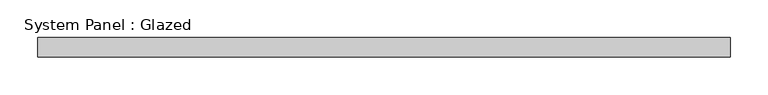
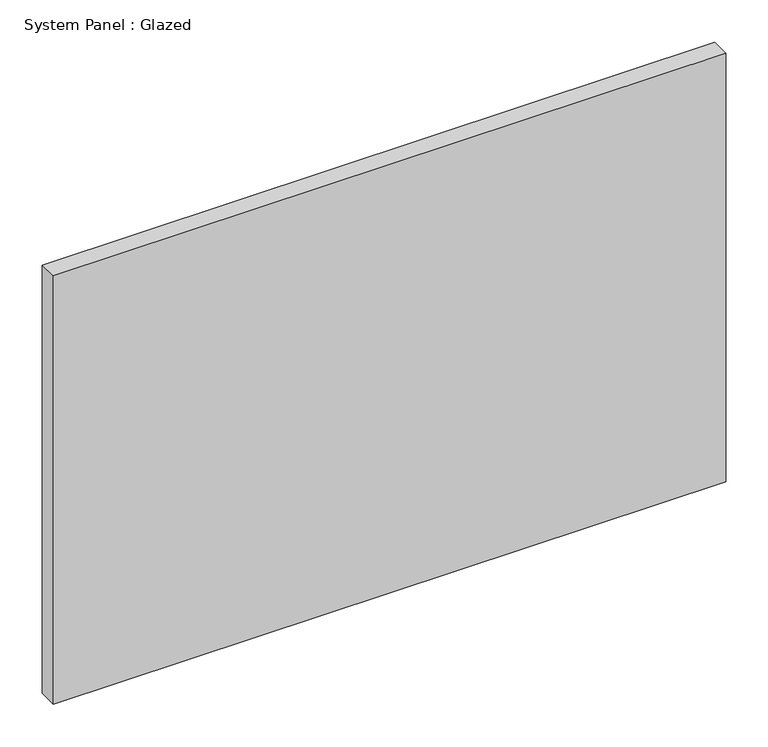
"""IFC4 building model written with IfcOpenShell, lengths in millimetres: plate geometry, System Panel : Glazed."""

from ifc_helpers import new_model, si_unit, origin, origin_with_axes, place, context, project, spatial, polyline, outline, extrude, source, transform, mapped, element, save


def system_panel_glazed_7d1a27c5(model_context):
    return source(origin(), model_context, "Body", "SweptSolid", [
        extrude(outline(polyline([(457.2, 19.05), (-457.2, 19.05), (-457.2, 44.45), (457.2, 44.45), (457.2, 19.05)])), origin_with_axes(), (0.0, 0.0, 1.0), 615.95),
    ])


if __name__ == "__main__":
    model = new_model("IFC4")
    model_context = context("Model", 3, world=origin())
    ifc_project = project(units=[si_unit("LENGTHUNIT", "METRE", prefix="MILLI")], contexts=[model_context])
    site = spatial("IfcSite", under=ifc_project)
    building = spatial("IfcBuilding", under=site)
    placement = place(None, origin())
    system_panel_glazed_shape = system_panel_glazed_7d1a27c5(model_context)
    element("IfcPlate", 1, ObjectType="System Panel : Glazed", at=placement, inside=building, context=model_context, shape_type="MappedRepresentation", body=[
        mapped(system_panel_glazed_shape, transform((0.0, 0.0, 0.0), x_axis=(1.0, 0.0, 0.0), y_axis=(0.0, 1.0, 0.0), z_axis=(0.0, 0.0, 1.0))),
    ])
    save(model, "model.ifc")

# Revit data of these elements
# Type "System Panel : Glazed"
#   Construction Type Id = "GSP4R"
#   Analytic Construction = "1/8 in Pilkington single glazing"
#   Visual Light Transmittance = 0.9
#   Solar Heat Gain Coefficient = 0.86
#   Heat Transfer Coefficient (U) = 1.18115 BTU/(h·ft²·°F)
# Element 1 (IfcPlate, "System Panel : Glazed")
#   Materials on its faces: "Glass"
# Materials
#   "Glass": class "Glass", colour RGB 0 128 192, transparency 0.75, Description = "Soda Lime Glass", Cost = 0
